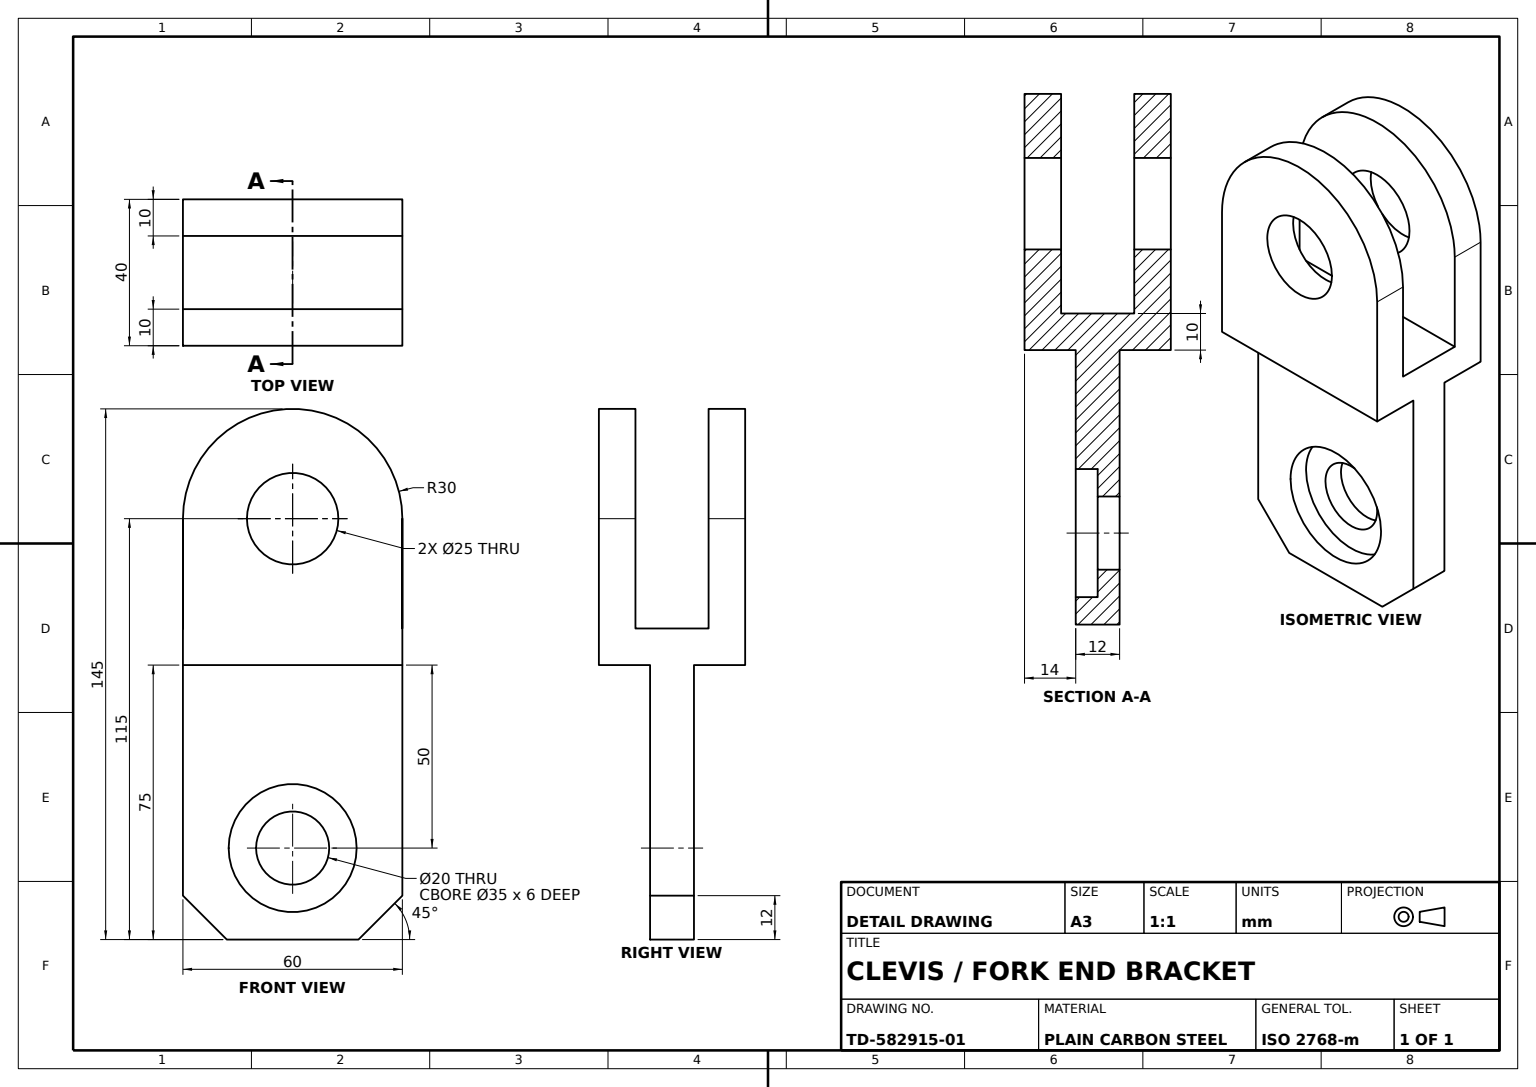
SolidWorks part; units mm, degrees
material "Plain Carbon Steel"
ref_plane "Front Plane" through (0, 0, 0) normal (0, 0, 1) x (1, 0, 0)
ref_plane "Top Plane" through (0, 0, 0) normal (0, 1, 0) x (1, 0, 0)
ref_plane "Right Plane" through (0, 0, 0) normal (1, 0, 0) x (0, 0, -1)
sketch "Base Plate Profile" plane through (0, 0, 0) normal (0, 0, 1) x (1, 0, 0)
  line L1 (-6, 0) -> (-6, -63)
  line L4 (-6, -63) -> (6, -75)
  line L5 (6, -75) -> (42, -75)
  line L6 (54, -63) -> (54, 0)
  line L10 (54, -63) -> (42, -75)
  line L11 (-6, 0) -> (54, 0)
  dimension "D1" = 60
  dimension "D2" = 63
  dimension "D3" = 12
  dimension "D4" = 75
  dimension "D5" = 12
  dimension "D6" = 6
extrude "Base Plate" add sketch "Base Plate Profile" along normal blind 12
sketch "Clevis Body Profile" plane through (-6, 0, 0) normal (-1, 0, 0) x (0, 0, 1)
  line L0 (12, 0) -> (26, 0)
  line L1 (26, 0) -> (26, 40)
  line L2 (26, 40) -> (12, 40)
  line L3 (12, 40) -> (12, 0)
  line L4 (0, 0) -> (-14, 0)
  line L5 (-14, 0) -> (-14, 40)
  line L6 (-14, 40) -> (0, 40)
  line L7 (0, 40) -> (0, 0)
  dimension "D1" = 40
  dimension "D2" = 14
  dimension "D3" = 14
extrude "Clevis Body" add sketch "Clevis Body Profile" against normal blind 60
sketch "Lug 1 Boss Sketch" plane through (0, 0, -14) normal (0, 0, -1) x (-1, 0, 0)
  line L0 (-54, 40) -> (6, 40) construction
  circle A0 centre (-24, 40) radius 30
  dimension "D1" = 60
extrude "Lug 1 Boss" add sketch "Lug 1 Boss Sketch" against normal blind 10
sketch "Lug 1 Trim Sketch" plane through (0, 40, 0) normal (0, 1, 0) x (1, 0, 0)
  line L0 (-6, 4) -> (54, 4)
  line L1 (54, 4) -> (54, 0)
  line L2 (54, 0) -> (-6, 0)
  line L3 (-6, 0) -> (-6, 4)
extrude "Lug 1 Trim" cut sketch "Lug 1 Trim Sketch" against normal blind 40
sketch "Lug 2 Boss Sketch" plane through (0, 0, 26) normal (0, 0, 1) x (1, 0, 0)
  line L0 (54, 40) -> (-6, 40) construction
  circle A0 centre (24, 40) radius 30
  dimension "D1" = 60
extrude "Lug 2 Boss" add sketch "Lug 2 Boss Sketch" against normal blind 10
sketch "Lug 2 Trim Sketch" plane through (0, 40, 0) normal (0, 1, 0) x (1, 0, 0)
  line L0 (-6, -12) -> (-6, -16)
  line L1 (-6, -16) -> (54, -16)
  line L2 (54, -16) -> (54, -12)
  line L3 (54, -12) -> (-6, -12)
extrude "Lug 2 Trim" cut sketch "Lug 2 Trim Sketch" against normal blind 40
sketch "Clevis Web Sketch" plane through (0, 0, 0) normal (0, 1, 0) x (1, 0, 0)
  line L0 (-6, 4) -> (54, 4)
  line L1 (54, 4) -> (54, -16)
  line L2 (54, -16) -> (-6, -16)
  line L3 (-6, -16) -> (-6, 4)
extrude "Clevis Web" add sketch "Clevis Web Sketch" along normal blind 10
sketch "Pin Hole Sketch" plane through (0, 0, 26) normal (0, 0, 1) x (1, 0, 0)
  circle A0 centre (24, 40) radius 12.5
  dimension "D1" = 25
  dimension "D2" = 25
extrude "Pin Hole Ø25" cut sketch "Pin Hole Sketch" against normal blind 40
sketch "Counterbore Sketch" plane through (0, 0, 12) normal (0, 0, 1) x (1, 0, 0)
  line L0 (-6, 0) -> (-6, -63) construction
  line L1 (54, 0) -> (-6, 0) construction
  circle A0 centre (24, -50) radius 17.5
  dimension "D1" = 35
  dimension "D2" = 35
  dimension "D3" = 30
  dimension "D4" = 50
extrude "Counterbore Ø35x6" cut sketch "Counterbore Sketch" against normal blind 6
sketch "Mounting Hole Sketch" plane through (0, 0, 6) normal (0, 0, 1) x (1, 0, 0)
  circle A0 centre (24, -50) radius 10
  dimension "D1" = 20
  dimension "D2" = 20
extrude "Mounting Hole Ø20" cut sketch "Mounting Hole Sketch" against normal blind 6
